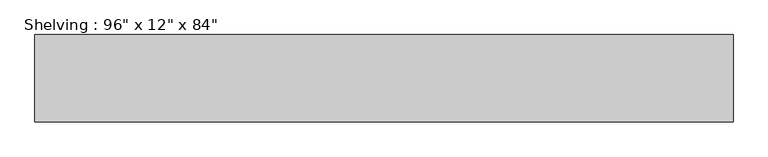
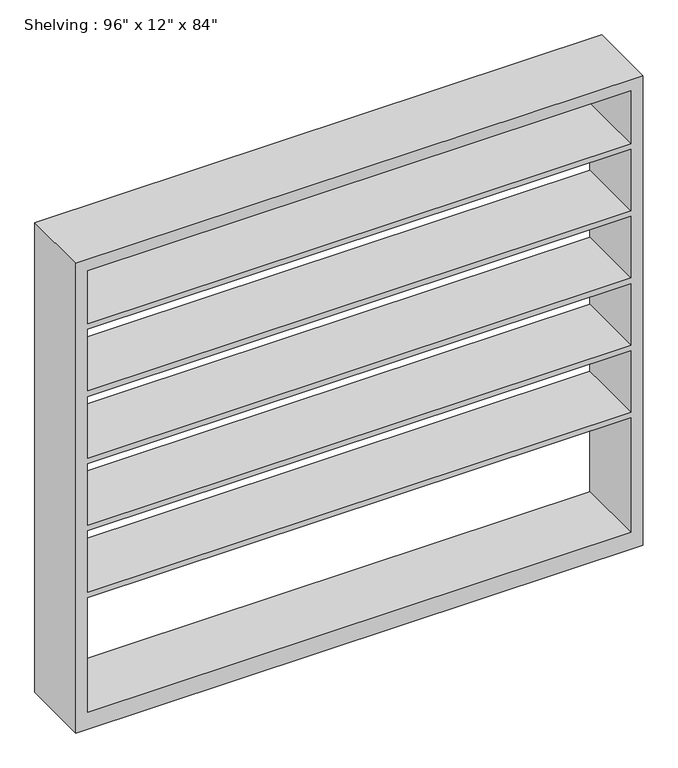
"""IFC4 building model written with IfcOpenShell, lengths in millimetres: furniture geometry."""

from ifc_helpers import new_model, si_unit, frame, origin, place, context, project, spatial, polyline, outline, extrude, source, transform, mapped, element, save


def furniture_b1da5ad0(model_context):
    return source(origin(), model_context, "Body", "SweptSolid", [
        extrude(outline(polyline([(0.0, 1219.2), (2133.6, 1219.2), (2133.6, -1219.2), (0.0, -1219.2), (0.0, 1219.2)]), holes=[polyline([(2082.8, 1168.4), (1841.5, 1168.4), (1841.5, -1168.4), (2082.8, -1168.4), (2082.8, 1168.4)]), polyline([(76.2, 1168.4), (76.2, -1168.4), (596.9, -1168.4), (596.9, 1168.4), (76.2, 1168.4)]), polyline([(1231.9, -1168.4), (1511.3, -1168.4), (1511.3, 1168.4), (1231.9, 1168.4), (1231.9, -1168.4)]), polyline([(1816.1, 1168.4), (1536.7, 1168.4), (1536.7, -1168.4), (1816.1, -1168.4), (1816.1, 1168.4)]), polyline([(1206.5, 1168.4), (927.1, 1168.4), (927.1, -1168.4), (1206.5, -1168.4), (1206.5, 1168.4)]), polyline([(901.7, 1168.4), (622.3, 1168.4), (622.3, -1168.4), (901.7, -1168.4), (901.7, 1168.4)])]), frame((0.0, -457.2, 0.0), z_axis=(0.0, 1.0, 0.0), x_axis=(0.0, 0.0, 1.0)), (0.0, 0.0, 1.0), 304.8),
    ])


if __name__ == "__main__":
    model = new_model("IFC4")
    model_context = context("Model", 3, world=origin())
    ifc_project = project(units=[si_unit("LENGTHUNIT", "METRE", prefix="MILLI")], contexts=[model_context])
    site = spatial("IfcSite", under=ifc_project)
    building = spatial("IfcBuilding", under=site)
    placement = place(None, origin())
    furniture_shape = furniture_b1da5ad0(model_context)
    element("IfcFurniture", 1, ObjectType="Shelving : 96\" x 12\" x 84\"", at=placement, inside=building, context=model_context, shape_type="MappedRepresentation", body=[
        mapped(furniture_shape, transform((0.0, 0.0, 0.0), x_axis=(1.0, 0.0, 0.0), y_axis=(0.0, 1.0, 0.0), z_axis=(0.0, 0.0, 1.0))),
    ])
    save(model, "model.ifc")

# Revit data of these elements
# Type "Shelving : 96\" x 12\" x 84\""
#   Assembly Code = "E2020200"
#   Depth = 1' - 0"
#   Height = 7' - 0"
#   Width = 8' - 0"
#   Shelving Unit Material = Laminate, Ivory, Matte
#   Default Elevation = 0
# Element 1 (IfcFurniture, "Shelving : 96\" x 12\" x 84\"")
#   Materials on its faces: "Laminate, Ivory, Matte"
# Materials
#   "Laminate, Ivory, Matte": class "Plastic", colour RGB 247 247 239, transparency 0, Description = "Plastic Laminate - Ivory, Matte", Cost = 0
